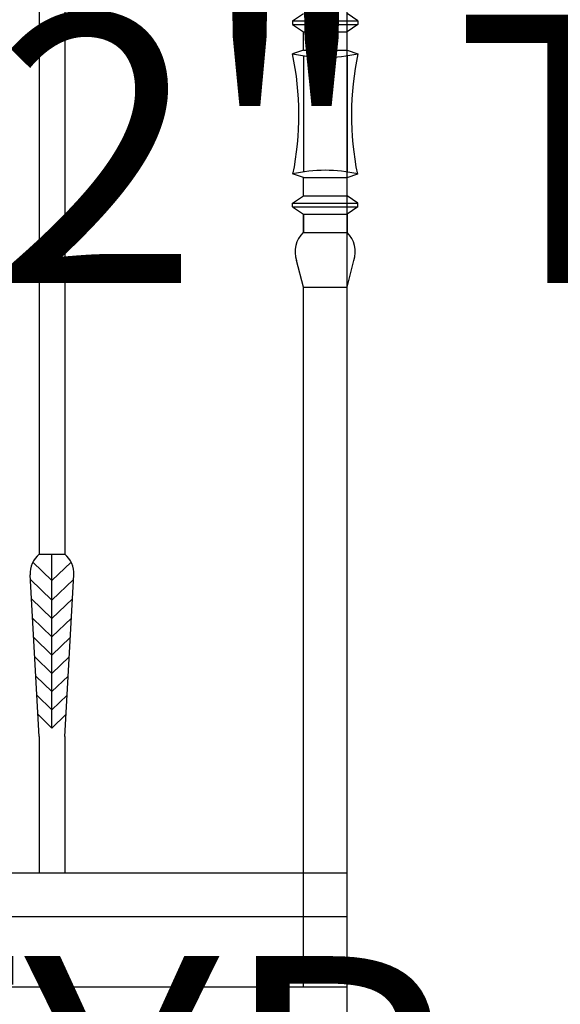
# Model space of a CAD drawing. Units: inches. Extents: x 2278 to 7495, y -71 to 1198.
# Tile 34 of 44: x 5138.35 to 5150.45, y 123.86 to 145.88. Entities that reach past the tile are written whole.
import ezdxf

# ---------------------------------------------------------------- set-up
doc = ezdxf.new("R2010")
doc.units = ezdxf.units.IN
doc.header["$MEASUREMENT"] = 0
doc.layers.add('A-ANNO-DIMS', color=2, linetype='Continuous', lineweight=18)
doc.layers.add('A-ELEV', color=7, linetype='Continuous', lineweight=25)
doc.styles.get("Standard").update_dxf_attribs({"font": 'arial.ttf'})
doc.dimstyles.get("Standard").update_dxf_attribs({"dimtxt": 6, "dimasz": 3, "dimexe": 0.18, "dimexo": 0.0625, "dimgap": 0.09, "dimtad": 0, "dimtih": 1, "dimtoh": 1, "dimdec": 0, "dimzin": 0, "dimdsep": 46, "dimlunit": 3, "dimtxsty": 'Standard', "dimblk": 'ARCHTICK', "dimcen": 0.09, "dimadec": 0, "dimazin": 0, "dimtfac": 1, "dimtdec": 0, "dimtofl": 0, "dimtmove": 0, "dimatfit": 3, "dimfxl": 1, "dimtolj": 1, "dimtzin": 0, "dimarcsym": 0})

# ---------------------------------------------------------------- blocks, each defined once
blk = doc.blocks.new('_ArchTick')
at = {"color": 0, "linetype": 'ByBlock', "const_width": 0.15}
blk.add_lwpolyline([(-0.5, -0.5), (0.5, 0.5)], dxfattribs=at)
blk = doc.blocks.new('*D59')
at = {"layer": 'A-ANNO-DIMS', "color": 0, "lineweight": -2, "transparency": 16777216}
for p, q in [((5096.589, 159.183), (5101.564, 159.183)), ((5101.384, 159.183), (5101.384, 146.185)), ((5101.384, 126.799), (5101.384, 139.796)), ((5096.589, 126.799), (5101.564, 126.799))]:
    blk.add_line(p, q, dxfattribs=at)
at = {"layer": 'Defpoints', "color": 0, "transparency": 16777216}
for p in [(5096.527, 159.183), (5101.384, 159.183), (5096.527, 126.799)]:
    blk.add_point(p, dxfattribs=at)
at = {"layer": 'A-ANNO-DIMS', "color": 0, "lineweight": -2, "transparency": 16777216, "xscale": 3, "yscale": 3, "zscale": 3}
for p, rotation in [((5101.384, 159.183), 90), ((5101.384, 126.799), 270)]:
    blk.add_blockref('_ArchTick', p, dxfattribs=dict(at, rotation=rotation))
at = {"layer": 'A-ANNO-DIMS', "color": 0, "transparency": 16777216, "insert": (5101.384, 142.991), "char_height": 6, "attachment_point": 5}
blk.add_mtext('\\A1;ORNATE BALUSTER 2\'-8 1/2" TYP.', dxfattribs=at)
blk = doc.blocks.new('*D60')
at = {"layer": 'A-ANNO-DIMS', "color": 0, "lineweight": -2, "transparency": 16777216}
for p, q in [((5088.787, 126.736), (5088.787, 121.761)), ((5096.527, 126.736), (5096.527, 121.761)), ((5088.787, 121.941), (5096.527, 121.941)), ((5096.527, 121.941), (5099.527, 121.941))]:
    blk.add_line(p, q, dxfattribs=at)
at = {"layer": 'Defpoints', "color": 0, "transparency": 16777216}
for p in [(5088.787, 126.799), (5096.527, 126.799), (5096.527, 121.941)]:
    blk.add_point(p, dxfattribs=at)
at = {"layer": 'A-ANNO-DIMS', "color": 0, "lineweight": -2, "transparency": 16777216, "xscale": 3, "yscale": 3, "zscale": 3, "rotation": 180}
blk.add_blockref('_ArchTick', (5088.787, 121.941), dxfattribs=at)
at = {"layer": 'A-ANNO-DIMS', "color": 0, "lineweight": -2, "transparency": 16777216, "xscale": 3, "yscale": 3, "zscale": 3}
blk.add_blockref('_ArchTick', (5096.527, 121.941), dxfattribs=at)
at = {"layer": 'A-ANNO-DIMS', "color": 0, "transparency": 16777216, "insert": (5124.894, 121.941), "char_height": 6, "attachment_point": 5}
blk.add_mtext('\\A1;0\'-7 1/2" TYP.', dxfattribs=at)
blk = doc.blocks.new('*D123')
at = {"layer": 'A-ANNO-DIMS', "color": 0, "lineweight": -2, "transparency": 16777216}
for p, q in [((4736.95, 340.157), (4736.95, -23.427)), ((5145.676, -1.81), (5145.676, -23.427)), ((4736.95, -23.247), (4923.929, -23.247)), ((5145.676, -23.247), (4958.697, -23.247))]:
    blk.add_line(p, q, dxfattribs=at)
at = {"layer": 'Defpoints', "color": 0, "transparency": 16777216}
for p in [(4736.95, 340.219), (5145.676, -1.747), (5145.676, -23.247)]:
    blk.add_point(p, dxfattribs=at)
at = {"layer": 'A-ANNO-DIMS', "color": 0, "lineweight": -2, "transparency": 16777216, "xscale": 3, "yscale": 3, "zscale": 3, "rotation": 180}
blk.add_blockref('_ArchTick', (4736.95, -23.247), dxfattribs=at)
at = {"layer": 'A-ANNO-DIMS', "color": 0, "lineweight": -2, "transparency": 16777216, "xscale": 3, "yscale": 3, "zscale": 3}
blk.add_blockref('_ArchTick', (5145.676, -23.247), dxfattribs=at)
at = {"layer": 'A-ANNO-DIMS', "color": 0, "transparency": 16777216, "insert": (4941.313, -23.247), "char_height": 6, "attachment_point": 5}
blk.add_mtext('\\A1;34\'-0 1/2"', dxfattribs=at)
blk = doc.blocks.new('*D131')
at = {"layer": 'A-ANNO-DIMS', "color": 0, "lineweight": -2, "transparency": 16777216}
for p, q in [((5096.176, 99.315), (5096.176, 361.899)), ((5145.676, 118.315), (5145.676, 361.899)), ((5096.176, 361.719), (5105.75, 361.719)), ((5145.676, 361.719), (5136.102, 361.719))]:
    blk.add_line(p, q, dxfattribs=at)
at = {"layer": 'Defpoints', "color": 0, "transparency": 16777216}
for p in [(5145.676, 361.719), (5145.676, 118.253), (5096.176, 99.253)]:
    blk.add_point(p, dxfattribs=at)
at = {"layer": 'A-ANNO-DIMS', "color": 0, "lineweight": -2, "transparency": 16777216, "xscale": 3, "yscale": 3, "zscale": 3, "rotation": 180}
blk.add_blockref('_ArchTick', (5096.176, 361.719), dxfattribs=at)
at = {"layer": 'A-ANNO-DIMS', "color": 0, "lineweight": -2, "transparency": 16777216, "xscale": 3, "yscale": 3, "zscale": 3}
blk.add_blockref('_ArchTick', (5145.676, 361.719), dxfattribs=at)
at = {"layer": 'A-ANNO-DIMS', "color": 0, "transparency": 16777216, "insert": (5120.926, 361.719), "char_height": 6, "attachment_point": 5}
blk.add_mtext('\\A1;4\'-1 1/2"', dxfattribs=at)
blk = doc.blocks.new('*D139')
at = {"layer": 'A-ANNO-DIMS', "color": 0, "lineweight": -2, "transparency": 16777216}
for p, q in [((5092.239, 160.253), (5167.754, 160.253)), ((5167.574, 160.253), (5167.574, 142.408)), ((5167.574, 118.253), (5167.574, 136.097)), ((5145.739, 118.253), (5167.754, 118.253))]:
    blk.add_line(p, q, dxfattribs=at)
at = {"layer": 'Defpoints', "color": 0, "transparency": 16777216}
for p in [(5092.176, 160.253), (5167.574, 160.253), (5145.676, 118.253)]:
    blk.add_point(p, dxfattribs=at)
at = {"layer": 'A-ANNO-DIMS', "color": 0, "lineweight": -2, "transparency": 16777216, "xscale": 3, "yscale": 3, "zscale": 3}
for p, rotation in [((5167.574, 160.253), 90), ((5167.574, 118.253), 270)]:
    blk.add_blockref('_ArchTick', p, dxfattribs=dict(at, rotation=rotation))
at = {"layer": 'A-ANNO-DIMS', "color": 0, "transparency": 16777216, "insert": (5167.574, 139.253), "char_height": 6, "attachment_point": 5}
blk.add_mtext('\\A1;3\'-6"', dxfattribs=at)
blk = doc.blocks.new('*D144')
at = {"layer": 'A-ANNO-DIMS', "color": 0, "lineweight": -2, "transparency": 16777216}
for p, q in [((5145.739, 244.253), (5167.754, 244.253)), ((5167.574, 244.253), (5167.574, 184.406)), ((5167.574, 118.253), (5167.574, 178.099)), ((5145.739, 118.253), (5167.754, 118.253))]:
    blk.add_line(p, q, dxfattribs=at)
at = {"layer": 'Defpoints', "color": 0, "transparency": 16777216}
for p in [(5145.676, 244.253), (5167.574, 244.253), (5145.676, 118.253)]:
    blk.add_point(p, dxfattribs=at)
at = {"layer": 'A-ANNO-DIMS', "color": 0, "lineweight": -2, "transparency": 16777216, "xscale": 3, "yscale": 3, "zscale": 3}
for p, rotation in [((5167.574, 244.253), 90), ((5167.574, 118.253), 270)]:
    blk.add_blockref('_ArchTick', p, dxfattribs=dict(at, rotation=rotation))
at = {"layer": 'A-ANNO-DIMS', "color": 0, "transparency": 16777216, "insert": (5167.574, 181.253), "char_height": 6, "attachment_point": 5}
blk.add_mtext('\\A1;10\'-6"', dxfattribs=at)

msp = doc.modelspace()

# ---------------------------------------------------------------- linework, layer by layer
at = {"layer": 'A-ELEV'}
for p, q in [((5145.676, -1.747), (5145.676, 161.577)), ((5138.792, 148.728), (5138.792, 133.927)), ((5139.362, 148.728), (5139.362, 133.927)), ((5144.454, 145.849), (5144.699, 146.012)), ((5145.921, 145.849), (5145.676, 146.012)), ((5144.454, 145.849), (5145.921, 145.849)), ((5144.454, 145.849), (5144.454, 145.768)), ((5144.454, 145.768), (5145.921, 145.768)), ((5144.454, 145.768), (5144.699, 145.605)), ((5145.921, 145.768), (5145.676, 145.605)), ((5145.921, 145.849), (5145.921, 145.768)), ((5144.699, 145.198), (5144.699, 145.605)), ((5144.699, 145.605), (5145.676, 145.605)), ((5145.676, 145.198), (5145.676, 145.605)), ((5144.699, 145.198), (5144.454, 145.116)), ((5144.699, 145.198), (5145.676, 145.198)), ((5144.699, 145.07), (5144.699, 142.474)), ((5145.676, 145.198), (5145.921, 145.116)), ((5145.676, 145.07), (5145.676, 142.474)), ((5144.699, 142.346), (5144.454, 142.428)), ((5145.676, 142.346), (5145.921, 142.428)), ((5144.699, 142.346), (5145.676, 142.346)), ((5144.699, 141.936), (5144.699, 142.346)), ((5145.676, 141.936), (5145.676, 142.346)), ((5144.454, 141.773), (5144.699, 141.936)), ((5144.454, 141.773), (5145.921, 141.773)), ((5144.454, 141.691), (5144.454, 141.773)), ((5144.699, 141.936), (5145.676, 141.936)), ((5145.921, 141.773), (5145.676, 141.936)), ((5145.921, 141.691), (5145.921, 141.773)), ((5144.454, 141.691), (5145.921, 141.691)), ((5144.454, 141.691), (5144.699, 141.529)), ((5145.921, 141.691), (5145.676, 141.529)), ((5144.699, 141.529), (5145.676, 141.529)), ((5144.699, 141.121), (5144.699, 141.529)), ((5144.699, 141.529), (5144.699, 141.121)), ((5145.676, 141.121), (5145.676, 141.529)), ((5145.676, 141.529), (5145.676, 141.121)), ((5144.699, 141.121), (5145.676, 141.121)), ((5144.699, 139.899), (5144.546, 140.492)), ((5145.676, 139.899), (5145.829, 140.492)), ((5144.699, 124.253), (5144.699, 139.899)), ((5144.699, 139.899), (5145.676, 139.899)), ((5145.676, 124.253), (5145.676, 139.899)), ((5138.792, 133.927), (5139.362, 133.927)), ((5139.077, 130.039), (5139.077, 133.927)), ((5138.649, 133.751), (5139.077, 133.337)), ((5139.506, 133.751), (5139.077, 133.337)), ((5138.792, 129.854), (5138.59, 133.463)), ((5139.362, 129.854), (5139.564, 133.463)), ((5138.596, 133.361), (5139.077, 132.896)), ((5139.559, 133.361), (5139.077, 132.896)), ((5138.62, 132.93), (5139.077, 132.488)), ((5139.535, 132.93), (5139.077, 132.488)), ((5138.644, 132.498), (5139.077, 132.079)), ((5139.51, 132.498), (5139.077, 132.079)), ((5138.668, 132.067), (5139.077, 131.671)), ((5139.486, 132.067), (5139.077, 131.671)), ((5138.692, 131.635), (5139.077, 131.263)), ((5139.462, 131.635), (5139.077, 131.263)), ((5138.716, 131.204), (5139.077, 130.855)), ((5139.438, 131.204), (5139.077, 130.855)), ((5138.741, 130.772), (5139.077, 130.447)), ((5139.414, 130.772), (5139.077, 130.447)), ((5138.765, 130.341), (5139.077, 130.039)), ((5139.39, 130.341), (5139.077, 130.039)), ((5138.792, 129.854), (5138.792, 126.799)), ((5139.362, 129.854), (5139.362, 126.799)), ((5145.676, 126.799), (5066.016, 126.799)), ((5145.676, 125.821), (5066.016, 125.821)), ((4874.676, 124.253), (5145.676, 124.253))]:
    msp.add_line(p, q, dxfattribs=at)
for centre, radius, start, end in [((5138.084, 143.743), 6.517, 348.3176, 12.1601), ((5145.187, 148.339), 3.305, 257.1818, 282.8182), ((5152.291, 143.743), 6.517, 167.8399, 191.6824), ((5145.187, 139.205), 3.305, 77.1818, 102.8182), ((5145.122, 140.685), 0.608, 134.1319, 198.5268), ((5145.253, 140.685), 0.608, 341.4732, 45.8681), ((5139.136, 133.502), 0.547, 128.9283, 183.9822), ((5139.018, 133.502), 0.547, 356.0178, 51.0717)]:
    msp.add_arc(centre, radius, start, end, dxfattribs=at)

# ---------------------------------------------------------------- dimensions: what is measured, and where the dimension line sits
at = {"layer": 'A-ANNO-DIMS'}
for base, p1, p2, picture, middle in [((5145.676, 361.719), (5096.176, 99.253), (5145.676, 118.253), '*D131', (5120.926, 361.719)), ((5145.676, -23.247), (4736.95, 340.219), (5145.676, -1.747), '*D123', (4941.313, -23.247))]:
    dim = msp.add_linear_dim(base=base, p1=p1, p2=p2, dimstyle='Standard', override={"dimdec": 1, "dimlfac": 1, "dimrnd": 0, "dimzin": 1, "dimdsep": 46, "dimlunit": 4, "dimfrac": 2}, dxfattribs=at)
    dim.commit()
    dim.dimension.update_dxf_attribs({"geometry": picture, "text_midpoint": middle})
for base, p2, picture, middle in [((5167.574, 244.253), (5145.676, 244.253), '*D144', (5167.574, 181.253)), ((5167.574, 160.253), (5092.176, 160.253), '*D139', (5167.574, 139.253))]:
    dim = msp.add_linear_dim(base=base, p1=(5145.676, 118.253), p2=p2, angle=90, dimstyle='Standard', override={"dimdec": 1, "dimlfac": 1, "dimrnd": 0, "dimzin": 1, "dimdsep": 46, "dimlunit": 4, "dimfrac": 2}, dxfattribs=at)
    dim.commit()
    dim.dimension.update_dxf_attribs({"geometry": picture, "text_midpoint": middle})
dim = msp.add_linear_dim(base=(5101.384, 159.183), p1=(5096.527, 126.799), p2=(5096.527, 159.183), angle=90, text='ORNATE BALUSTER <> TYP.', dimstyle='Standard', override={"dimdec": 1, "dimrnd": 0, "dimzin": 1, "dimlunit": 4, "dimfrac": 2}, dxfattribs=at)
dim.commit()
dim.dimension.update_dxf_attribs({"geometry": '*D59', "text_midpoint": (5101.384, 142.991)})
dim = msp.add_linear_dim(base=(5096.527, 121.941), p1=(5088.787, 126.799), p2=(5096.527, 126.799), text='<> TYP.', dimstyle='Standard', override={"dimdec": 1, "dimrnd": 0, "dimzin": 1, "dimlunit": 4, "dimfrac": 2}, dxfattribs=at)
dim.commit()
dim.dimension.update_dxf_attribs({"geometry": '*D60', "text_midpoint": (5124.894, 121.941)})

doc.saveas('drawing.dxf')
